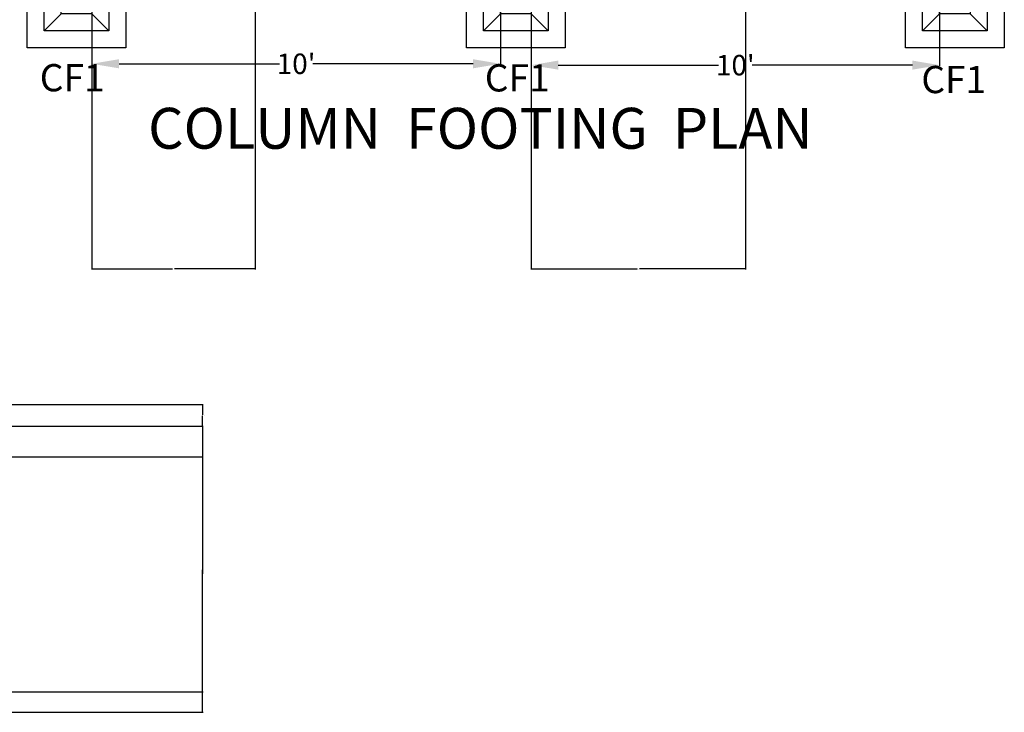
# Model space of a CAD drawing. Units: inches. Extents: x 37 to 824, y -700 to 234.
# Tile 22 of 77: x 503 to 792, y -580 to -377. Entities that reach past the tile are written whole.
import ezdxf

# ---------------------------------------------------------------- set-up
doc = ezdxf.new("R2010")
doc.units = ezdxf.units.IN
doc.header["$MEASUREMENT"] = 0
for name, color, linetype, lineweight in [('A-ANNO-DIMS', 2, 'Continuous', 18), ('A-ANNO-TEXT', 7, 'Continuous', 18), ('S-FNDN', 220, 'Continuous', 25)]:
    doc.layers.add(name, color=color, linetype=linetype, lineweight=lineweight)
doc.styles.get("Standard").update_dxf_attribs({"font": 'arial.ttf'})
doc.dimstyles.get("Standard").update_dxf_attribs({"dimtxt": 0.18, "dimasz": 0.18, "dimexe": 0.18, "dimexo": 0.0625, "dimgap": 0.09, "dimtad": 0, "dimtih": 1, "dimtoh": 1, "dimdec": 1, "dimzin": 0, "dimdsep": 46, "dimlunit": 4, "dimtxsty": 'Standard', "dimcen": 0.09, "dimadec": 0, "dimazin": 0, "dimtfac": 1, "dimtdec": 1, "dimtofl": 0, "dimtmove": 0, "dimatfit": 3, "dimfxl": 1, "dimtolj": 1, "dimtzin": 0, "dimarcsym": 0})

# ---------------------------------------------------------------- blocks, each defined once
blk = doc.blocks.new('*D24')
at = {"layer": 'A-ANNO-DIMS', "color": 0, "lineweight": -2, "ltscale": 0.5, "transparency": 16777216}
for p, q in [((524.2, -365.97), (524.2, -389.77)), ((644.2, -365.97), (644.2, -389.77)), ((532.2, -389.59), (579.3, -389.59)), ((636.2, -389.59), (589.1, -389.59))]:
    blk.add_line(p, q, dxfattribs=at)
at = {"layer": 'A-ANNO-DIMS', "color": 0, "ltscale": 0.5, "transparency": 16777216}
for points in [[(532.2, -388.25), (532.2, -390.92), (524.2, -389.59)], [(636.2, -388.25), (636.2, -390.92), (644.2, -389.59)]]:
    blk.add_solid(points, dxfattribs=at)
at = {"layer": 'Defpoints', "color": 0, "ltscale": 0.5, "transparency": 16777216}
for p in [(524.2, -365.91), (644.2, -365.91), (644.2, -389.59)]:
    blk.add_point(p, dxfattribs=at)
at = {"layer": 'A-ANNO-DIMS', "color": 0, "ltscale": 0.5, "transparency": 16777216, "insert": (584.2, -389.59), "char_height": 6, "attachment_point": 5}
blk.add_mtext("\\A1;10'", dxfattribs=at)
blk = doc.blocks.new('*D25')
at = {"layer": 'A-ANNO-DIMS', "color": 0, "lineweight": -2, "ltscale": 0.5, "transparency": 16777216}
for p, q in [((653.2, -365.97), (653.2, -390.17)), ((773.2, -365.97), (773.2, -390.17)), ((661.2, -389.99), (708.3, -389.99)), ((765.2, -389.99), (718.1, -389.99))]:
    blk.add_line(p, q, dxfattribs=at)
at = {"layer": 'A-ANNO-DIMS', "color": 0, "ltscale": 0.5, "transparency": 16777216}
for points in [[(661.2, -388.65), (661.2, -391.32), (653.2, -389.99)], [(765.2, -388.65), (765.2, -391.32), (773.2, -389.99)]]:
    blk.add_solid(points, dxfattribs=at)
at = {"layer": 'Defpoints', "color": 0, "ltscale": 0.5, "transparency": 16777216}
for p in [(653.2, -365.91), (773.2, -365.91), (773.2, -389.99)]:
    blk.add_point(p, dxfattribs=at)
at = {"layer": 'A-ANNO-DIMS', "color": 0, "ltscale": 0.5, "transparency": 16777216, "insert": (713.2, -389.99), "char_height": 6, "attachment_point": 5}
blk.add_mtext("\\A1;10'", dxfattribs=at)
blk = doc.blocks.new('FOOTING-CF1')
at = {"ltscale": 0.6}
for p, q in [((0, 29), (29, 29)), ((0, 0), (0, 29)), ((29, 29), (29, 0)), ((29, 0), (0, 0))]:
    blk.add_line(p, q, dxfattribs=at)
for p, q in [((5, 24), (24, 24)), ((5, 5), (5, 24)), ((5, 24), (10, 19)), ((19, 19), (24, 24)), ((24, 24), (24, 5)), ((10, 19), (19, 19)), ((10, 10), (10, 19)), ((19, 19), (19, 10)), ((5, 5), (10, 10)), ((19, 10), (10, 10)), ((24, 5), (19, 10)), ((24, 5), (5, 5))]:
    blk.add_line(p, q)
blk = doc.blocks.new('*D90')
at = {"layer": 'A-ANNO-DIMS', "color": 0, "lineweight": -2, "ltscale": 0.5, "transparency": 16777216}
for p, q in [((524.2, -11.97), (524.2, -450)), ((572.2, -11.97), (572.2, -450)), ((524.38, -449.82), (547.87, -449.82)), ((572.02, -449.82), (548.53, -449.82))]:
    blk.add_line(p, q, dxfattribs=at)
at = {"layer": 'A-ANNO-DIMS', "color": 0, "ltscale": 0.5, "transparency": 16777216}
for points in [[(524.38, -449.79), (524.38, -449.85), (524.2, -449.82)], [(572.02, -449.79), (572.02, -449.85), (572.2, -449.82)]]:
    blk.add_solid(points, dxfattribs=at)
at = {"layer": 'Defpoints', "color": 0, "ltscale": 0.5, "transparency": 16777216}
for p in [(524.2, -11.91), (572.2, -11.91), (572.2, -449.82)]:
    blk.add_point(p, dxfattribs=at)
at = {"layer": 'A-ANNO-DIMS', "color": 0, "ltscale": 0.5, "transparency": 16777216, "insert": (548.2, -449.82), "char_height": 0.18, "attachment_point": 5}
blk.add_mtext('\\A1;4\'-0"', dxfattribs=at)
blk = doc.blocks.new('*D91')
at = {"layer": 'A-ANNO-DIMS', "color": 0, "lineweight": -2, "ltscale": 0.5, "transparency": 16777216}
for p, q in [((653.2, 66.03), (653.2, -450)), ((716.2, 66.03), (716.2, -450)), ((653.38, -449.82), (684.37, -449.82)), ((716.02, -449.82), (685.03, -449.82))]:
    blk.add_line(p, q, dxfattribs=at)
at = {"layer": 'A-ANNO-DIMS', "color": 0, "ltscale": 0.5, "transparency": 16777216}
for points in [[(653.38, -449.79), (653.38, -449.85), (653.2, -449.82)], [(716.02, -449.79), (716.02, -449.85), (716.2, -449.82)]]:
    blk.add_solid(points, dxfattribs=at)
at = {"layer": 'Defpoints', "color": 0, "ltscale": 0.5, "transparency": 16777216}
for p in [(653.2, 66.09), (716.2, 66.09), (716.2, -449.82)]:
    blk.add_point(p, dxfattribs=at)
at = {"layer": 'A-ANNO-DIMS', "color": 0, "ltscale": 0.5, "transparency": 16777216, "insert": (684.7, -449.82), "char_height": 0.18, "attachment_point": 5}
blk.add_mtext('\\A1;5\'-3"', dxfattribs=at)
blk = doc.blocks.new('*D100')
at = {"layer": 'A-ANNO-DIMS', "color": 0, "lineweight": -2, "ltscale": 0.5, "transparency": 16777216}
for p, q in [((358.19, -489.63), (556.92, -489.63)), ((556.74, -489.81), (556.74, -492.63)), ((556.74, -495.83), (556.74, -493)), ((348.26, -496.01), (556.92, -496.01))]:
    blk.add_line(p, q, dxfattribs=at)
at = {"layer": 'A-ANNO-DIMS', "color": 0, "ltscale": 0.5, "transparency": 16777216}
for points in [[(556.71, -489.81), (556.77, -489.81), (556.74, -489.63)], [(556.71, -495.83), (556.77, -495.83), (556.74, -496.01)]]:
    blk.add_solid(points, dxfattribs=at)
at = {"layer": 'Defpoints', "color": 0, "ltscale": 0.5, "transparency": 16777216}
for p in [(358.13, -489.63), (348.2, -496.01), (556.74, -496.01)]:
    blk.add_point(p, dxfattribs=at)
at = {"layer": 'A-ANNO-DIMS', "color": 0, "ltscale": 0.5, "transparency": 16777216, "insert": (556.74, -492.82), "char_height": 0.18, "attachment_point": 5}
blk.add_mtext('\\A1;0\'-6 1/2"', dxfattribs=at)
blk = doc.blocks.new('*D101')
at = {"layer": 'A-ANNO-DIMS', "color": 0, "lineweight": -2, "ltscale": 0.5, "transparency": 16777216}
for p, q in [((348.26, -496.01), (556.92, -496.01)), ((556.74, -496.19), (556.74, -537.82)), ((556.74, -579.83), (556.74, -538.19)), ((348.26, -580.01), (556.92, -580.01))]:
    blk.add_line(p, q, dxfattribs=at)
at = {"layer": 'A-ANNO-DIMS', "color": 0, "ltscale": 0.5, "transparency": 16777216}
for points in [[(556.71, -496.19), (556.77, -496.19), (556.74, -496.01)], [(556.71, -579.83), (556.77, -579.83), (556.74, -580.01)]]:
    blk.add_solid(points, dxfattribs=at)
at = {"layer": 'Defpoints', "color": 0, "ltscale": 0.5, "transparency": 16777216}
for p in [(348.2, -496.01), (348.2, -580.01), (556.74, -580.01)]:
    blk.add_point(p, dxfattribs=at)
at = {"layer": 'A-ANNO-DIMS', "color": 0, "ltscale": 0.5, "transparency": 16777216, "insert": (556.74, -538.01), "char_height": 0.18, "attachment_point": 5}
blk.add_mtext('\\A1;7\'-0"', dxfattribs=at)
blk = doc.blocks.new('*D104')
at = {"layer": 'A-ANNO-DIMS', "color": 0, "lineweight": -2, "ltscale": 0.5, "transparency": 16777216}
for p, q in [((341.26, -505.03), (556.92, -505.03)), ((556.74, -505.21), (556.74, -539.34)), ((556.74, -573.83), (556.74, -539.7)), ((341.26, -574.01), (556.92, -574.01))]:
    blk.add_line(p, q, dxfattribs=at)
at = {"layer": 'A-ANNO-DIMS', "color": 0, "ltscale": 0.5, "transparency": 16777216}
for points in [[(556.71, -505.21), (556.77, -505.21), (556.74, -505.03)], [(556.71, -573.83), (556.77, -573.83), (556.74, -574.01)]]:
    blk.add_solid(points, dxfattribs=at)
at = {"layer": 'Defpoints', "color": 0, "ltscale": 0.5, "transparency": 16777216}
for p in [(341.2, -505.03), (341.2, -574.01), (556.74, -574.01)]:
    blk.add_point(p, dxfattribs=at)
at = {"layer": 'A-ANNO-DIMS', "color": 0, "ltscale": 0.5, "transparency": 16777216, "insert": (556.74, -539.52), "char_height": 0.18, "attachment_point": 5}
blk.add_mtext('\\A1;5\'-9"', dxfattribs=at)

msp = doc.modelspace()

# ---------------------------------------------------------------- block references
at = {"layer": 'S-FNDN'}
for p, rotation in [((505.2, -355.91), 269.9999999999995), ((663.2, -355.91), 180), ((792.2, -384.91), 90.00000000000104)]:
    msp.add_blockref('FOOTING-CF1', p, dxfattribs=dict(at, rotation=rotation))

# ---------------------------------------------------------------- texts
at = {"layer": 'A-ANNO-TEXT'}
for s, height, p in [('CF1', 8, (508.91, -397.68)), ('CF1', 8, (639.62, -397.72)), ('CF1', 8, (767.83, -398.21)), ('COLUMN  FOOTING  PLAN', 12, (540.72, -414.53))]:
    msp.add_text(s, height=height, dxfattribs=at).set_placement(p)

# ---------------------------------------------------------------- dimensions: what is measured, and where the dimension line sits
at = {"layer": 'A-ANNO-DIMS', "ltscale": 0.5}
for base, p1, p2, override, picture, middle in [((716.2, -449.82), (653.2, 66.09), (716.2, 66.09), {"dimdec": 1, "dimlfac": 1, "dimrnd": 0, "dimzin": 1, "dimdsep": 46, "dimlunit": 4, "dimfrac": 2}, '*D91', (684.7, -449.82)), ((572.2, -449.82), (524.2, -11.91), (572.2, -11.91), {"dimdec": 1, "dimlfac": 1, "dimrnd": 0, "dimzin": 1, "dimdsep": 46, "dimlunit": 4, "dimfrac": 2}, '*D90', (548.2, -449.82)), ((644.2, -389.59), (524.2, -365.91), (644.2, -365.91), {"dimtxt": 6, "dimasz": 8, "dimclrd": 0, "dimclre": 0, "dimclrt": 0}, '*D24', (584.2, -389.59)), ((773.2, -389.99), (653.2, -365.91), (773.2, -365.91), {"dimtxt": 6, "dimasz": 8, "dimclrd": 0, "dimclre": 0, "dimclrt": 0}, '*D25', (713.2, -389.99))]:
    dim = msp.add_linear_dim(base=base, p1=p1, p2=p2, dimstyle='Standard', override=override, dxfattribs=at)
    dim.commit()
    dim.dimension.update_dxf_attribs({"geometry": picture, "text_midpoint": middle})
for base, p1, p2, picture, middle in [((556.74, -496.01), (358.13, -489.63), (348.2, -496.01), '*D100', (556.74, -492.82)), ((556.74, -580.01), (348.2, -496.01), (348.2, -580.01), '*D101', (556.74, -538.01)), ((556.74, -574.01), (341.2, -505.03), (341.2, -574.01), '*D104', (556.74, -539.52))]:
    dim = msp.add_linear_dim(base=base, p1=p1, p2=p2, angle=90, dimstyle='Standard', override={"dimdec": 1, "dimlfac": 1, "dimrnd": 0, "dimzin": 1, "dimdsep": 46, "dimlunit": 4, "dimfrac": 2}, dxfattribs=at)
    dim.commit()
    dim.dimension.update_dxf_attribs({"geometry": picture, "text_midpoint": middle})

doc.saveas('drawing.dxf')
